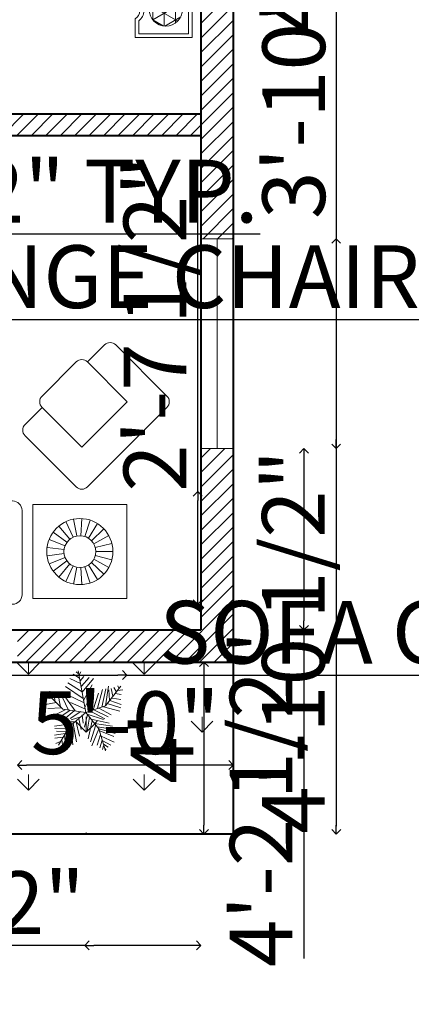
# Model space of a CAD drawing. Units: inches. Extents: x 597 to 1323, y 1833 to 2686.
# Tile 3 of 10: x 1048 to 1158, y 1896 to 2171. Entities that reach past the tile are written whole.
import ezdxf

# ---------------------------------------------------------------- set-up
doc = ezdxf.new("R2010")
doc.units = ezdxf.units.IN
for name, color, linetype, lineweight in [('A-ANNO-DIMS', 2, 'Continuous', 18), ('A-GLAZ', 2, 'Continuous', 18), ('A-WALL', 7, 'Continuous', 40), ('A-WALL-PATT', 8, 'Continuous', 13), ('BEDS', 6, 'Continuous', 18), ('L-PLNT', 3, 'Continuous', 18), ('L-PLNT-PATT', 3, 'Continuous', 13), ('SOFA', 10, 'Continuous', 18)]:
    doc.layers.add(name, color=color, linetype=linetype, lineweight=lineweight)
doc.styles.get("Standard").update_dxf_attribs({"font": 'arial.ttf'})
doc.dimstyles.new('ISO-25', dxfattribs={"dimtxt": 17.5, "dimasz": 2.5, "dimexe": 0, "dimexo": 0, "dimtad": 1, "dimdec": 1, "dimlunit": 3, "dimtxsty": 'Standard', "dimblk": 'OPEN90', "dimcen": 2.5, "dimadec": 0, "dimazin": 0, "dimtfac": 1, "dimtdec": 1, "dimtmove": 0, "dimatfit": 3, "dimfxl": 0, "dimfxlon": 1, "dimarcsym": 0})

# ---------------------------------------------------------------- blocks, each defined once
blk = doc.blocks.new('new block')
for p, q in [((-74.3, 8.91), (-74.3, 27.23)), ((-56.5, 8.91), (-56.5, 27.23)), ((-119.59, 17.47), (-120.49, 22.18)), ((-118.48, 17.54), (-118.18, 22.32)), ((-13.95, 17.47), (-14.85, 22.18)), ((-12.84, 17.54), (-12.54, 22.32)), ((-121.59, 16.53), (-124.64, 20.23)), ((-120.65, 17.13), (-122.69, 21.46)), ((-117.39, 17.33), (-115.91, 21.89)), ((-116.38, 16.86), (-113.82, 20.91)), ((-115.53, 16.15), (-112.03, 19.43)), ((-15.95, 16.53), (-19, 20.23)), ((-15.01, 17.13), (-17.05, 21.46)), ((-11.75, 17.33), (-10.27, 21.89)), ((-10.74, 16.86), (-8.17, 20.91)), ((-9.89, 16.15), (-6.39, 19.43)), ((-122.88, 14.75), (-127.34, 16.51)), ((-122.35, 15.72), (-126.23, 18.54)), ((-114.87, 15.25), (-110.67, 17.56)), ((-17.24, 14.75), (-21.7, 16.51)), ((-16.71, 15.72), (-20.59, 18.54)), ((-9.23, 15.25), (-5.03, 17.56)), ((-123.16, 13.67), (-127.92, 14.27)), ((-114.47, 14.22), (-109.82, 15.41)), ((-17.52, 13.67), (-22.27, 14.27)), ((-8.82, 14.22), (-4.18, 15.41)), ((-123.16, 12.56), (-127.92, 11.96)), ((-122.88, 11.48), (-127.34, 9.72)), ((-114.47, 12.01), (-109.82, 10.82)), ((-114.33, 13.11), (-109.53, 13.11)), ((-17.52, 12.56), (-22.27, 11.96)), ((-17.24, 11.48), (-21.7, 9.72)), ((-8.82, 12.01), (-4.18, 10.82)), ((-8.68, 13.11), (-3.89, 13.11)), ((-122.35, 10.51), (-126.23, 7.69)), ((-121.59, 9.7), (-124.64, 6)), ((-120.65, 9.1), (-122.69, 4.76)), ((-119.59, 8.76), (-120.49, 4.05)), ((-118.48, 8.69), (-118.18, 3.9)), ((-117.39, 8.9), (-115.91, 4.34)), ((-116.38, 9.37), (-113.82, 5.32)), ((-115.53, 10.08), (-112.03, 6.8)), ((-114.87, 10.98), (-110.67, 8.67)), ((-16.71, 10.51), (-20.59, 7.69)), ((-15.95, 9.7), (-19, 6)), ((-15.01, 9.1), (-17.05, 4.76)), ((-13.95, 8.76), (-14.85, 4.05)), ((-12.84, 8.69), (-12.54, 3.9)), ((-11.75, 8.9), (-10.27, 4.34)), ((-10.74, 9.37), (-8.17, 5.32)), ((-9.89, 10.08), (-6.39, 6.8)), ((-9.23, 10.98), (-5.03, 8.67))]:
    blk.add_line(p, q)
blk.add_lwpolyline([(-56.5, 27.23, 0.414214), (-59.12, 29.85), (-71.69, 29.85, 0.414214), (-74.3, 27.23, 0.414214), (-76.92, 29.85), (-89.49, 29.85, 0.414214), (-92.11, 27.23), (-92.11, 8.91), (-39.75, 8.91), (-39.75, 27.23, 0.414214), (-42.36, 29.85), (-53.88, 29.85, 0.414214)], format="xyb", close=True)
for points in [[(-131.88, 26.23), (-105.64, 26.23), (-105.64, 0), (-131.88, 0)], [(-26.24, 26.23), (0, 26.23), (0, 0), (-26.24, 0)]]:
    blk.add_lwpolyline(points, close=True)
blk.add_lwpolyline([(-92.11, 27.23), (-99.96, 27.23, 0.414214), (-102.58, 24.61), (-102.58, 1.05, 0.414214), (-99.96, -1.57), (-31.89, -1.57, 0.414214), (-29.27, 1.05), (-29.27, 24.61, 0.414214), (-31.89, 27.23), (-39.75, 27.23)], format="xyb")
for centre, radius in [((-118.76, 13.11), 9.23), ((-13.12, 13.11), 9.23), ((-118.76, 13.11), 4.43), ((-13.12, 13.11), 4.43)]:
    blk.add_circle(centre, radius)
blk = doc.blocks.new('*U2')
for p, q in [((-10.186, 53.64), (-13.084, 55.962)), ((0, 0), (-10.5, 57)), ((-9.099, 51.782), (-6.563, 55.962)), ((-5.114, 28.097), (-24.676, 40.636)), ((-7.288, 39.707), (-21.778, 46.673)), ((-8.737, 47.138), (-17.069, 52.711)), ((-7.65, 43.423), (-2.578, 49.46)), ((-5.839, 35.992), (4.667, 48.067)), ((-5.114, 27.632), (10.463, 46.673)), ((-48.585, 21.131), (-49.309, 29.026)), ((-43.513, 28.561), (-42.427, 15.558)), ((-35.544, 28.097), (-24.314, 3.947)), ((-3.665, 19.273), (-27.574, 35.527)), ((-2.941, 16.486), (8.652, 37.85)), ((16.259, 5.805), (23.142, 31.348)), ((22.055, 7.198), (27.489, 32.277)), ((27, 9), (48, 36)), ((27.127, 9.056), (31.112, 35.992)), ((31.836, 30.883), (32.561, 16.486)), ((35.096, 32.741), (37.27, 22.524)), ((38.719, 34.134), (41.979, 28.561)), ((43.791, 29.954), (51.036, 30.883)), ((44.153, 36.456), (45.239, 32.741)), ((-47.498, 19.737), (-55.83, 18.344)), ((-40.615, 13.7), (-55.105, 10.913)), ((-31.5, 4.5), (-52.5, 25.5)), ((-38.442, 26.239), (-34.819, 7.663)), ((-14.533, 2.09), (-30.834, 25.31)), ((-24.314, 23.917), (-2.941, 13.7)), ((-20.691, 13.7), (-1.129, 4.876)), ((-1.129, 6.734), (9.014, 26.704)), ((3.942, 1.625), (11.187, 24.381)), ((10.101, 3.483), (17.708, 26.239)), ((33.285, 16.486), (48.862, 10.913)), ((36.183, 19.737), (48.137, 17.88)), ((40.53, 25.775), (48.862, 24.846)), ((-33.37, 6.269), (-52.207, 5.34)), ((-28.299, 3.483), (-47.86, -5.805)), ((-21.416, 3.018), (-38.079, -8.128)), ((0, 0), (-31.5, 4.5)), ((-15.982, 2.09), (-30.11, -9.521)), ((0, 0), (-22.5, -19.5)), ((-6.563, 1.161), (-21.416, -8.128)), ((0, 0), (27, 9)), ((0, 0), (18, -22.5)), ((6.478, 1.625), (26.04, -8.592)), ((11.187, 3.483), (30.749, -5.805)), ((18.07, 5.805), (35.096, -3.483)), ((24.229, 7.663), (46.688, 1.625)), ((29.662, 12.307), (48.137, 6.269)), ((-15.257, -12.772), (-30.11, -12.772)), ((-6.563, -5.805), (-19.967, -9.985)), ((-13.446, -11.378), (-8.737, -32.741)), ((-9.461, -8.592), (-6.201, -23.453)), ((-4.752, -3.483), (-3.665, -14.629)), ((2.493, -3.019), (-1.491, -20.202)), ((1.769, -2.555), (24.229, -9.521)), ((5.029, -6.27), (2.131, -25.775)), ((9.014, -11.378), (3.58, -35.992)), ((7.565, -9.056), (32.198, -14.629)), ((-17.431, -15.094), (-42.789, -18.809)), ((-24.314, -21.596), (-42.427, -22.06)), ((-26.849, -26.24), (-40.253, -25.775)), ((-22.5, -19.5), (-37.5, -45)), ((-25.038, -23.918), (-22.865, -45.281)), ((-20.691, -18.345), (-17.793, -44.352)), ((-17.069, -15.094), (-12.721, -40.172)), ((14.085, -16.951), (6.478, -40.172)), ((18.07, -22.524), (8.289, -45.745)), ((12.274, -15.094), (36.907, -18.809)), ((16.259, -19.738), (36.183, -22.989)), ((18, -22.5), (27, -52.5)), ((18.433, -22.524), (40.53, -29.026)), ((19.157, -25.311), (38.719, -33.206)), ((-28.299, -29.026), (-42.789, -31.348)), ((-30.834, -34.135), (-42.427, -35.528)), ((-34.457, -39.708), (-40.978, -42.494)), ((-32.646, -36.921), (-31.921, -44.352)), ((-29.023, -30.884), (-27.936, -43.887)), ((20.244, -30.419), (15.897, -44.816)), ((22.78, -37.85), (19.519, -48.532)), ((21.331, -32.741), (39.081, -40.636)), ((22.78, -38.314), (34.372, -44.816)), ((24.591, -45.745), (23.142, -50.854)), ((24.591, -43.423), (30.749, -47.603)), ((26.764, -49.925), (28.213, -50.854))]:
    blk.add_line(p, q)
blk = doc.blocks.new('_Open90')
at = {"color": 0, "linetype": 'ByBlock', "lineweight": -2}
for p, q in [((0, 0), (-1, 0)), ((-0.5, 0.5), (0, 0)), ((0, 0), (-0.5, -0.5))]:
    blk.add_line(p, q, dxfattribs=at)
blk = doc.blocks.new('*D22')
at = {"layer": 'A-ANNO-DIMS', "color": 0, "lineweight": -2, "transparency": 16777216}
blk.add_line((1136.67, 2421.11), (1136.67, 1946.11), dxfattribs=at)
at = {"layer": 'Defpoints', "color": 0, "transparency": 16777216}
for p in [(1107.89, 2423.61), (1107.89, 1943.61), (1136.67, 1943.61)]:
    blk.add_point(p, dxfattribs=at)
at = {"layer": 'A-ANNO-DIMS', "color": 0, "lineweight": -2, "transparency": 16777216, "xscale": 2.5, "yscale": 2.5, "zscale": 2.5}
for p, rotation in [((1136.67, 2423.61), 90), ((1136.67, 1943.61), 270)]:
    blk.add_blockref('_Open90', p, dxfattribs=dict(at, rotation=rotation))
at = {"layer": 'A-ANNO-DIMS', "color": 0, "transparency": 16777216, "insert": (1127.11, 2183.61), "char_height": 17.5, "attachment_point": 5, "rotation": 90}
blk.add_mtext("40'", dxfattribs=at)
blk = doc.blocks.new('*D23')
at = {"layer": 'A-ANNO-DIMS', "color": 0, "lineweight": -2, "transparency": 16777216}
blk.add_line((1099.7, 1989.11), (1099.7, 1946.11), dxfattribs=at)
at = {"layer": 'Defpoints', "color": 0, "transparency": 16777216}
for p in [(1107.89, 1991.61), (1099.7, 1943.61), (1107.89, 1943.61)]:
    blk.add_point(p, dxfattribs=at)
at = {"layer": 'A-ANNO-DIMS', "color": 0, "lineweight": -2, "transparency": 16777216, "xscale": 2.5, "yscale": 2.5, "zscale": 2.5}
for p, rotation in [((1099.7, 1991.61), 90), ((1099.7, 1943.61), 270)]:
    blk.add_blockref('_Open90', p, dxfattribs=dict(at, rotation=rotation))
at = {"layer": 'A-ANNO-DIMS', "color": 0, "transparency": 16777216, "insert": (1090.32, 1967.61), "char_height": 17.5, "attachment_point": 5, "rotation": 90}
blk.add_mtext("4'", dxfattribs=at)
blk = doc.blocks.new('NIGHTSTAND')
h = blk.add_hatch()
h.set_pattern_fill('NET3', color=256)
h.set_pattern_definition([(0, (-854.688, -2394.344), (0, 3.175), []), (60, (-854.688, -2394.344), (-2.7496307, 1.5875), []), (120, (-854.688, -2394.344), (-2.7496307, -1.5875), [])])
h.paths.add_polyline_path([(12.33, 8.55, 1), (2.97, 8.55, 1)])
for points in [[(5.9, 0), (0, 0), (0, 15.92), (15.5, 15.92), (15.5, 0), (10.29, 0, 0.602187)], [(5.24, 1), (1, 1), (1, 14.92), (14.5, 14.92), (14.5, 1), (10.87, 1, 0.518163)]]:
    blk.add_lwpolyline(points, format="xyb", close=True)
blk.add_circle((7.65, 8.55), 4.68)
blk = doc.blocks.new('LOUNGE-CHAIR')
blk.add_lwpolyline([(18.09, 35.52), (22.84, 40.28, -0.414214), (26.01, 40.28), (40.28, 26.01, -0.414214), (40.28, 22.84), (18.09, 0.66, -0.414214), (14.92, 0.66), (0.66, 14.92, -0.414214), (0.66, 18.09), (5.41, 22.84)], format="xyb")
blk.add_lwpolyline([(5.41, 26.01), (14.92, 35.52, -0.414214), (18.09, 35.52), (29.18, 24.43), (16.5, 11.75), (5.41, 22.84, -0.414214)], format="xyb", close=True)
blk = doc.blocks.new('*D40')
at = {"layer": 'A-ANNO-DIMS', "color": 0, "lineweight": -2, "transparency": 16777216}
for p, q in [((941.18, 2111.08), (961.47, 2111.08)), ((963.97, 2111.08), (1115.46, 2111.08))]:
    blk.add_line(p, q, dxfattribs=at)
at = {"layer": 'Defpoints', "color": 0, "transparency": 16777216}
for p in [(938.68, 2115.46), (963.97, 2115.46), (963.97, 2111.08)]:
    blk.add_point(p, dxfattribs=at)
at = {"layer": 'A-ANNO-DIMS', "color": 0, "lineweight": -2, "transparency": 16777216, "xscale": 2.5, "yscale": 2.5, "zscale": 2.5, "rotation": 180}
blk.add_blockref('_Open90', (938.68, 2111.08), dxfattribs=at)
at = {"layer": 'A-ANNO-DIMS', "color": 0, "lineweight": -2, "transparency": 16777216, "xscale": 2.5, "yscale": 2.5, "zscale": 2.5}
blk.add_blockref('_Open90', (963.97, 2111.08), dxfattribs=at)
at = {"layer": 'A-ANNO-DIMS', "color": 0, "transparency": 16777216, "insert": (1040.96, 2120.76), "char_height": 17.5, "attachment_point": 5}
blk.add_mtext('2\'-1 1/2" TYP.', dxfattribs=at)
blk = doc.blocks.new('*D43')
at = {"layer": 'A-ANNO-DIMS', "color": 0, "lineweight": -2, "transparency": 16777216}
for p, q in [((939.8, 2087.21), (976.17, 2087.21)), ((978.67, 2087.21), (1321.98, 2087.21))]:
    blk.add_line(p, q, dxfattribs=at)
at = {"layer": 'Defpoints', "color": 0, "transparency": 16777216}
for p in [(978.67, 2087.21), (937.3, 2081.01), (978.67, 2081.01)]:
    blk.add_point(p, dxfattribs=at)
at = {"layer": 'A-ANNO-DIMS', "color": 0, "lineweight": -2, "transparency": 16777216, "xscale": 2.5, "yscale": 2.5, "zscale": 2.5, "rotation": 180}
blk.add_blockref('_Open90', (937.3, 2087.21), dxfattribs=at)
at = {"layer": 'A-ANNO-DIMS', "color": 0, "lineweight": -2, "transparency": 16777216, "xscale": 2.5, "yscale": 2.5, "zscale": 2.5}
blk.add_blockref('_Open90', (978.67, 2087.21), dxfattribs=at)
at = {"layer": 'A-ANNO-DIMS', "color": 0, "transparency": 16777216, "insert": (1151.58, 2096.9), "char_height": 17.5, "attachment_point": 5}
blk.add_mtext('LOUNGE CHAIR 3\'-5 1/2" TYP.', dxfattribs=at)
blk = doc.blocks.new('*D51')
at = {"layer": 'A-ANNO-DIMS', "color": 0, "lineweight": -2, "transparency": 16777216}
for p, q in [((948.81, 1987.99), (1075.69, 1987.99)), ((1078.19, 1987.99), (1311.77, 1987.99))]:
    blk.add_line(p, q, dxfattribs=at)
at = {"layer": 'Defpoints', "color": 0, "transparency": 16777216}
for p in [(946.31, 2007.77), (1078.19, 2007.77), (1078.19, 1987.99)]:
    blk.add_point(p, dxfattribs=at)
at = {"layer": 'A-ANNO-DIMS', "color": 0, "lineweight": -2, "transparency": 16777216, "xscale": 2.5, "yscale": 2.5, "zscale": 2.5, "rotation": 180}
blk.add_blockref('_Open90', (946.31, 1987.99), dxfattribs=at)
at = {"layer": 'A-ANNO-DIMS', "color": 0, "lineweight": -2, "transparency": 16777216, "xscale": 2.5, "yscale": 2.5, "zscale": 2.5}
blk.add_blockref('_Open90', (1078.19, 1987.99), dxfattribs=at)
at = {"layer": 'A-ANNO-DIMS', "color": 0, "transparency": 16777216, "insert": (1196.23, 1997.67), "char_height": 17.5, "attachment_point": 5}
blk.add_mtext('SOFA GROUP 11\'-0"', dxfattribs=at)
blk = doc.blocks.new('*D52')
at = {"layer": 'A-ANNO-DIMS', "color": 0, "lineweight": -2, "transparency": 16777216}
for p, q in [((1097.98, 2039.19), (1097.98, 2130.53)), ((1097.98, 2010.27), (1097.98, 2036.69))]:
    blk.add_line(p, q, dxfattribs=at)
at = {"layer": 'Defpoints', "color": 0, "transparency": 16777216}
for p in [(1078.19, 2039.19), (1097.98, 2039.19), (1078.19, 2007.77)]:
    blk.add_point(p, dxfattribs=at)
at = {"layer": 'A-ANNO-DIMS', "color": 0, "lineweight": -2, "transparency": 16777216, "xscale": 2.5, "yscale": 2.5, "zscale": 2.5}
for p, rotation in [((1097.98, 2039.19), 90), ((1097.98, 2007.77), 270)]:
    blk.add_blockref('_Open90', p, dxfattribs=dict(at, rotation=rotation))
at = {"layer": 'A-ANNO-DIMS', "color": 0, "transparency": 16777216, "insert": (1088.3, 2086.11), "char_height": 17.5, "attachment_point": 5, "rotation": 90}
blk.add_mtext('2\'-7 1/2"', dxfattribs=at)
blk = doc.blocks.new('*D65')
at = {"layer": 'A-ANNO-DIMS', "color": 0, "lineweight": -2, "transparency": 16777216}
for p, q in [((1136.64, 2225.03), (1136.64, 2183.94)), ((1136.64, 2181.44), (1136.64, 2117.59))]:
    blk.add_line(p, q, dxfattribs=at)
at = {"layer": 'Defpoints', "color": 0, "transparency": 16777216}
for p in [(1107.89, 2227.53), (1107.89, 2181.44), (1136.64, 2181.44)]:
    blk.add_point(p, dxfattribs=at)
at = {"layer": 'A-ANNO-DIMS', "color": 0, "lineweight": -2, "transparency": 16777216, "xscale": 2.5, "yscale": 2.5, "zscale": 2.5}
for p, rotation in [((1136.64, 2227.53), 90), ((1136.64, 2181.44), 270)]:
    blk.add_blockref('_Open90', p, dxfattribs=dict(at, rotation=rotation))
at = {"layer": 'A-ANNO-DIMS', "color": 0, "transparency": 16777216, "insert": (1127.07, 2148.27), "char_height": 17.5, "attachment_point": 5, "rotation": 90}
blk.add_mtext('3\'-10"', dxfattribs=at)
blk = doc.blocks.new('*D66')
at = {"layer": 'A-ANNO-DIMS', "color": 0, "lineweight": -2, "transparency": 16777216}
for p, q in [((1136.64, 2107.26), (1136.64, 2053.7)), ((1136.64, 2051.2), (1136.64, 1945.85))]:
    blk.add_line(p, q, dxfattribs=at)
at = {"layer": 'Defpoints', "color": 0, "transparency": 16777216}
for p in [(1107.89, 2109.76), (1107.89, 2051.2), (1136.64, 2051.2)]:
    blk.add_point(p, dxfattribs=at)
at = {"layer": 'A-ANNO-DIMS', "color": 0, "lineweight": -2, "transparency": 16777216, "xscale": 2.5, "yscale": 2.5, "zscale": 2.5}
for p, rotation in [((1136.64, 2109.76), 90), ((1136.64, 2051.2), 270)]:
    blk.add_blockref('_Open90', p, dxfattribs=dict(at, rotation=rotation))
at = {"layer": 'A-ANNO-DIMS', "color": 0, "transparency": 16777216, "insert": (1126.96, 1997.28), "char_height": 17.5, "attachment_point": 5, "rotation": 90}
blk.add_mtext('4\'-10 1/2"', dxfattribs=at)
blk = doc.blocks.new('*D70')
at = {"layer": 'A-ANNO-DIMS', "color": 0, "lineweight": -2, "transparency": 16777216}
for p, q in [((1066.43, 1912.53), (975.08, 1912.53)), ((1096.39, 1912.53), (1068.93, 1912.53))]:
    blk.add_line(p, q, dxfattribs=at)
at = {"layer": 'Defpoints', "color": 0, "transparency": 16777216}
for p in [(1066.43, 2310.73), (1098.89, 2310.73), (1066.43, 1912.53)]:
    blk.add_point(p, dxfattribs=at)
at = {"layer": 'A-ANNO-DIMS', "color": 0, "lineweight": -2, "transparency": 16777216, "xscale": 2.5, "yscale": 2.5, "zscale": 2.5, "rotation": 180}
blk.add_blockref('_Open90', (1066.43, 1912.53), dxfattribs=at)
at = {"layer": 'A-ANNO-DIMS', "color": 0, "lineweight": -2, "transparency": 16777216, "xscale": 2.5, "yscale": 2.5, "zscale": 2.5}
blk.add_blockref('_Open90', (1098.89, 1912.53), dxfattribs=at)
at = {"layer": 'A-ANNO-DIMS', "color": 0, "transparency": 16777216, "insert": (1019.5, 1922.21), "char_height": 17.5, "attachment_point": 5}
blk.add_mtext('2\'-8 1/2"', dxfattribs=at)
blk = doc.blocks.new('*D75')
at = {"layer": 'A-ANNO-DIMS', "color": 0, "lineweight": -2, "transparency": 16777216}
for p, q in [((1127.64, 2048.7), (1127.64, 2003.11)), ((1127.64, 2000.61), (1127.64, 1908.86))]:
    blk.add_line(p, q, dxfattribs=at)
at = {"layer": 'Defpoints', "color": 0, "transparency": 16777216}
for p in [(1098.89, 2051.2), (1098.89, 2000.61), (1127.64, 2000.61)]:
    blk.add_point(p, dxfattribs=at)
at = {"layer": 'A-ANNO-DIMS', "color": 0, "lineweight": -2, "transparency": 16777216, "xscale": 2.5, "yscale": 2.5, "zscale": 2.5}
for p, rotation in [((1127.64, 2051.2), 90), ((1127.64, 2000.61), 270)]:
    blk.add_blockref('_Open90', p, dxfattribs=dict(at, rotation=rotation))
at = {"layer": 'A-ANNO-DIMS', "color": 0, "transparency": 16777216, "insert": (1117.96, 1953.48), "char_height": 17.5, "attachment_point": 5, "rotation": 90}
blk.add_mtext('4\'-2 1/2"', dxfattribs=at)
blk = doc.blocks.new('*D76')
at = {"layer": 'A-ANNO-DIMS', "color": 0, "lineweight": -2, "transparency": 16777216}
blk.add_line((1105.39, 1962.86), (1050.15, 1962.86), dxfattribs=at)
at = {"layer": 'Defpoints', "color": 0, "transparency": 16777216}
for p in [(1047.65, 1991.61), (1107.89, 1991.61), (1047.65, 1962.86)]:
    blk.add_point(p, dxfattribs=at)
at = {"layer": 'A-ANNO-DIMS', "color": 0, "lineweight": -2, "transparency": 16777216, "xscale": 2.5, "yscale": 2.5, "zscale": 2.5, "rotation": 180}
blk.add_blockref('_Open90', (1047.65, 1962.86), dxfattribs=at)
at = {"layer": 'A-ANNO-DIMS', "color": 0, "lineweight": -2, "transparency": 16777216, "xscale": 2.5, "yscale": 2.5, "zscale": 2.5}
blk.add_blockref('_Open90', (1107.89, 1962.86), dxfattribs=at)
at = {"layer": 'A-ANNO-DIMS', "color": 0, "transparency": 16777216, "insert": (1077.77, 1972.42), "char_height": 17.5, "attachment_point": 5}
blk.add_mtext('5\'-0"', dxfattribs=at)

msp = doc.modelspace()

# ---------------------------------------------------------------- hatches: boundary and pattern name
at = {"layer": 'A-WALL-PATT'}
h = msp.add_hatch(dxfattribs=at)
h.set_pattern_fill('ANSI31', color=256, scale=0.9)
h.paths.add_polyline_path([(927.93, 2423.61), (771.89, 2423.61), (771.89, 2371.61), (780.89, 2371.61), (780.89, 2414.61), (918.89, 2414.61), (927.93, 2414.61)])
h.paths.add_polyline_path([(1107.89, 2423.61), (1074.89, 2423.61), (1074.89, 2414.61), (1098.89, 2414.61), (1098.89, 2382.26), (1107.89, 2382.26)])
h.paths.add_polyline_path([(1002.89, 2423.61), (963.93, 2423.61), (963.93, 2414.61), (978.89, 2414.61), (1002.89, 2414.61)])
h.paths.add_polyline_path([(918.89, 2414.61), (912.89, 2414.61), (912.89, 2270.61), (906.2, 2270.61), (906.2, 2264.61), (918.89, 2264.61), (918.89, 2318.61), (928.09, 2318.61), (928.09, 2324.61), (918.89, 2324.61)])
h.paths.add_polyline_path([(780.89, 2299.61), (771.89, 2299.61), (771.89, 2245.99), (780.89, 2245.99)])
h.paths.add_polyline_path([(780.89, 2173.99), (771.89, 2173.99), (771.89, 1943.61), (790.26, 1943.61), (790.26, 1952.61), (780.89, 1952.61)])
h.paths.add_polyline_path([(873.89, 1991.61), (887.56, 1991.61), (887.56, 2000.61), (864.89, 2000.61), (864.89, 1952.61), (857.81, 1952.61), (857.81, 1943.61), (873.89, 1943.61)])
h.paths.add_polyline_path([(979.81, 2000.61), (908.62, 2000.61), (908.62, 1991.61), (979.81, 1991.61)])
h.paths.add_polyline_path([(931.89, 2138.61), (938.68, 2138.61), (938.68, 2144.61), (925.89, 2144.61), (925.89, 2000.61), (931.89, 2000.61)])
h.paths.add_polyline_path([(870.89, 2084.61), (874.89, 2084.61), (874.89, 2090.61), (870.89, 2090.61), (870.89, 2144.61), (815.52, 2144.61), (815.52, 2138.61), (864.89, 2138.61), (864.89, 2000.61), (870.89, 2000.61)])
h.paths.add_polyline_path([(925.89, 2090.61), (900.18, 2090.61), (900.18, 2084.61), (925.89, 2084.61)])
h.paths.add_polyline_path([(1107.89, 2051.2), (1098.89, 2051.2), (1098.89, 2000.61), (1047.65, 2000.61), (1047.65, 1991.61), (1107.89, 1991.61)])
h.paths.add_polyline_path([(1107.89, 2181.44), (1098.89, 2181.44), (1098.89, 2109.76), (1107.89, 2109.76)])
h.paths.add_polyline_path([(1098.89, 2144.61), (978.89, 2144.61), (978.89, 2157.94), (972.89, 2157.94), (972.89, 2144.61), (963.97, 2144.61), (963.97, 2138.61), (1098.89, 2138.61)])
h.paths.add_polyline_path([(1107.89, 2310.26), (1098.89, 2310.26), (1098.89, 2227.53), (1107.89, 2227.53)])
h.paths.add_polyline_path([(1098.89, 2270.61), (978.89, 2270.61), (978.89, 2276), (972.89, 2276), (972.89, 2183.23), (978.89, 2183.23), (978.89, 2264.61), (1098.89, 2264.61)])
h.paths.add_polyline_path([(880.92, 2270.61), (780.89, 2270.61), (780.89, 2264.61), (880.92, 2264.61)])
h.paths.add_polyline_path([(978.89, 2414.61), (972.89, 2414.61), (972.89, 2324.61), (961.07, 2324.61), (961.07, 2318.61), (972.89, 2318.61), (972.89, 2301.29), (978.89, 2301.29)])
h.paths.add_polyline_path([(790.26, 2144.61), (780.89, 2144.61), (780.89, 2138.61), (790.26, 2138.61)], flags=17)
at = {"layer": 'L-PLNT-PATT'}
h = msp.add_hatch(dxfattribs=at)
h.set_pattern_fill('GRASS', color=256, scale=0.9)
h.paths.add_polyline_path([(1107.89, 1991.61), (873.89, 1991.61), (873.89, 1943.61), (1107.89, 1943.61)])
h.paths.add_polyline_path([(897.46, 1969.81), (897.45, 1969.79), (897.46, 1969.78)], flags=16)
h.paths.add_polyline_path([(887.13, 1971.67), (886.91, 1971.63), (886.94, 1971.34)], flags=16)
h.paths.add_polyline_path([(891.46, 1976.37), (890.84, 1976.17), (890.9, 1975.88)], flags=16)
h.paths.add_polyline_path([(889.89, 1977.98), (889.78, 1978.14), (889.63, 1978.02)], flags=16)
h.paths.add_polyline_path([(890.92, 1987.98), (891.07, 1988.23), (890.84, 1988.41)], flags=16)
h.paths.add_polyline_path([(896.52, 1973), (896.51, 1972.97), (892.84, 1977.56), (894.89, 1978.24), (894.93, 1978.36), (895.05, 1978.3), (896.12, 1978.66), (896.19, 1978.92), (896.47, 1978.77), (898.33, 1979.39), (899.47, 1980.85), (899.46, 1980.97), (899.54, 1980.94), (898.36, 1979.43), (898.36, 1979.4), (892.84, 1977.56), (893.28, 1977.02), (893.36, 1976.99), (893.35, 1976.93), (894.3, 1975.74), (894.76, 1975.64), (894.68, 1975.27), (895.29, 1974.5), (895.81, 1974.42), (895.67, 1974.02), (896.48, 1973.02)], flags=16)
h.paths.add_polyline_path([(970.73, 1971.67), (970.51, 1971.63), (970.54, 1971.34)], flags=16)
h.paths.add_polyline_path([(973.49, 1977.98), (973.38, 1978.14), (973.23, 1978.02)], flags=16)
h.paths.add_polyline_path([(966.92, 1981.6), (966.59, 1981.54), (966.55, 1981.96), (969.68, 1978.84), (969.42, 1978.83), (969.35, 1979.16)], flags=16)
h.paths.add_polyline_path([(975.06, 1976.37), (974.44, 1976.17), (974.5, 1975.88)], flags=16)
h.paths.add_polyline_path([(974.52, 1987.98), (974.67, 1988.23), (974.44, 1988.41)], flags=16)
h.paths.add_polyline_path([(886.08, 1978.84), (885.82, 1978.83), (885.75, 1979.16), (883.32, 1981.6), (882.99, 1981.54), (882.95, 1981.96)], flags=16)
h.paths.add_polyline_path([(981.05, 1969.81), (981.05, 1969.79), (981.06, 1969.78)], flags=16)
h.paths.add_polyline_path([(976.44, 1977.56), (978.49, 1978.24), (978.52, 1978.36), (978.65, 1978.3), (979.72, 1978.66), (979.79, 1978.92), (980.06, 1978.77), (981.93, 1979.39), (983.06, 1980.85), (983.06, 1980.97), (983.14, 1980.94), (981.96, 1979.43), (981.96, 1979.4), (976.44, 1977.56), (976.87, 1977.02), (976.96, 1976.99), (976.94, 1976.93), (977.9, 1975.74), (978.36, 1975.64), (978.28, 1975.27), (978.89, 1974.5), (979.41, 1974.42), (979.27, 1974.02), (980.08, 1973.02), (980.12, 1973), (980.11, 1972.97)], flags=16)
h.paths.add_polyline_path([(1063.75, 1977.98), (1063.64, 1978.14), (1063.5, 1978.02)], flags=16)
h.paths.add_polyline_path([(1057.18, 1981.6), (1056.86, 1981.54), (1056.82, 1981.96), (1059.94, 1978.84), (1059.68, 1978.83), (1059.62, 1979.16)], flags=16)
h.paths.add_polyline_path([(1065.33, 1976.37), (1064.7, 1976.17), (1064.77, 1975.88)], flags=16)
h.paths.add_polyline_path([(1060.77, 1971.63), (1060.8, 1971.34), (1061, 1971.67)], flags=16)
h.paths.add_polyline_path([(1064.79, 1987.98), (1064.94, 1988.23), (1064.71, 1988.41)], flags=16)
h.paths.add_polyline_path([(1071.32, 1969.81), (1071.31, 1969.79), (1071.33, 1969.78)], flags=16)
h.paths.add_polyline_path([(1066.71, 1977.56), (1068.75, 1978.24), (1068.79, 1978.36), (1068.92, 1978.3), (1069.99, 1978.66), (1070.06, 1978.92), (1070.33, 1978.77), (1072.19, 1979.39), (1073.33, 1980.85), (1073.32, 1980.97), (1073.4, 1980.94), (1072.22, 1979.43), (1072.22, 1979.4), (1066.71, 1977.56), (1067.14, 1977.02), (1067.22, 1976.99), (1067.21, 1976.93), (1068.16, 1975.74), (1068.62, 1975.64), (1068.54, 1975.27), (1069.15, 1974.5), (1069.67, 1974.42), (1069.54, 1974.02), (1070.34, 1973.02), (1070.39, 1973), (1070.38, 1972.97)], flags=16)

# ---------------------------------------------------------------- linework, layer by layer
at = {"layer": 'A-GLAZ'}
for p, q in [((1098.89, 2109.76), (1107.89, 2109.76)), ((1103.39, 2109.76), (1103.39, 2051.2)), ((1098.89, 2051.2), (1107.89, 2051.2))]:
    msp.add_line(p, q, dxfattribs=at)
at = {"layer": 'A-WALL'}
for p, q in [((1107.89, 2423.61), (1107.89, 1943.61)), ((1098.89, 2414.61), (1098.89, 2000.61)), ((978.89, 2144.61), (1098.89, 2144.61)), ((963.97, 2138.61), (1098.89, 2138.61)), ((864.89, 2000.61), (1098.89, 2000.61)), ((873.89, 1991.61), (1107.89, 1991.61)), ((1107.89, 1943.61), (771.89, 1943.61))]:
    msp.add_line(p, q, dxfattribs=at)

# ---------------------------------------------------------------- block references
at = {"layer": 'BEDS', "rotation": 269.9999999999959}
msp.add_blockref('NIGHTSTAND', (1080.52, 2181.44), dxfattribs=at)
at = {"layer": 'L-PLNT', "xscale": 0.2033280951175252, "yscale": 0.2033280951175252, "zscale": 0.2033280951175252}
msp.add_blockref('*U2', (1066.71, 1977.56), dxfattribs=at)
at = {"layer": 'SOFA'}
for name, p in [('LOUNGE-CHAIR', (1049.11, 2039.85)), ('new block', (1078.19, 2009.34))]:
    msp.add_blockref(name, p, dxfattribs=at)

# ---------------------------------------------------------------- dimensions: what is measured, and where the dimension line sits
at = {"layer": 'A-ANNO-DIMS'}
for base, p1, p2, angle, override, picture, middle in [((1136.67, 1943.61), (1107.89, 2423.61), (1107.89, 1943.61), 90, {"dimclrd": 0, "dimclre": 0, "dimclrt": 0}, '*D22', (1127.11, 2183.61)), ((1136.64, 2181.44), (1107.89, 2227.53), (1107.89, 2181.44), 90, {"dimdec": 1, "dimlfac": 1, "dimrnd": 0, "dimzin": 1, "dimdsep": 46, "dimlunit": 4, "dimfrac": 2}, '*D65', (1127.07, 2148.27)), ((1097.98, 2039.19), (1078.19, 2007.77), (1078.19, 2039.19), 90, {"dimdec": 1, "dimlfac": 1, "dimrnd": 0, "dimzin": 1, "dimdsep": 46, "dimlunit": 4, "dimfrac": 2}, '*D52', (1088.3, 2086.11)), ((1136.64, 2051.2), (1107.89, 2109.76), (1107.89, 2051.2), 90, {"dimdec": 1, "dimlfac": 1, "dimrnd": 0, "dimzin": 1, "dimdsep": 46, "dimlunit": 4, "dimfrac": 2}, '*D66', (1126.96, 1997.28)), ((1127.64, 2000.61), (1098.89, 2051.2), (1098.89, 2000.61), 270, {"dimdec": 1, "dimlfac": 1, "dimrnd": 0, "dimzin": 1, "dimdsep": 46, "dimlunit": 4, "dimfrac": 2}, '*D75', (1117.96, 1953.48)), ((1047.65, 1962.86), (1107.89, 1991.61), (1047.65, 1991.61), 180, {"dimdec": 1, "dimlfac": 1, "dimrnd": 0, "dimzin": 1, "dimdsep": 46, "dimlunit": 4, "dimfrac": 2}, '*D76', (1077.77, 1972.42)), ((1099.7, 1943.61), (1107.89, 1991.61), (1107.89, 1943.61), 90, {"dimclrd": 0, "dimclre": 0, "dimclrt": 0}, '*D23', (1090.32, 1967.61))]:
    dim = msp.add_linear_dim(base=base, p1=p1, p2=p2, angle=angle, dimstyle='ISO-25', override=override, dxfattribs=at)
    dim.commit()
    dim.dimension.update_dxf_attribs({"geometry": picture, "text_midpoint": middle})
dim = msp.add_linear_dim(base=(1066.43, 1912.53), p1=(1098.89, 2310.73), p2=(1066.43, 2310.73), dimstyle='ISO-25', override={"dimdec": 1, "dimlfac": 1, "dimrnd": 0, "dimzin": 1, "dimdsep": 46, "dimlunit": 4, "dimfrac": 2}, dxfattribs=at)
dim.commit()
dim.dimension.update_dxf_attribs({"geometry": '*D70', "text_midpoint": (1019.5, 1922.21)})
for base, p1, p2, text, picture, middle in [((978.67, 2087.21), (937.3, 2081.01), (978.67, 2081.01), 'LOUNGE CHAIR <> TYP.', '*D43', (1151.58, 2096.9)), ((963.97, 2111.08), (938.68, 2115.46), (963.97, 2115.46), '<> TYP.', '*D40', (1040.96, 2120.76)), ((1078.19, 1987.99), (946.31, 2007.77), (1078.19, 2007.77), 'SOFA GROUP <>', '*D51', (1196.23, 1997.67))]:
    dim = msp.add_linear_dim(base=base, p1=p1, p2=p2, text=text, dimstyle='ISO-25', override={"dimdec": 1, "dimlfac": 1, "dimrnd": 0, "dimzin": 1, "dimdsep": 46, "dimlunit": 4, "dimfrac": 2}, dxfattribs=at)
    dim.commit()
    dim.dimension.update_dxf_attribs({"geometry": picture, "text_midpoint": middle})

doc.saveas('drawing.dxf')
